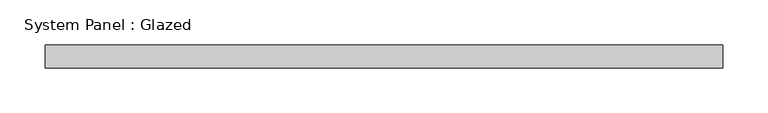
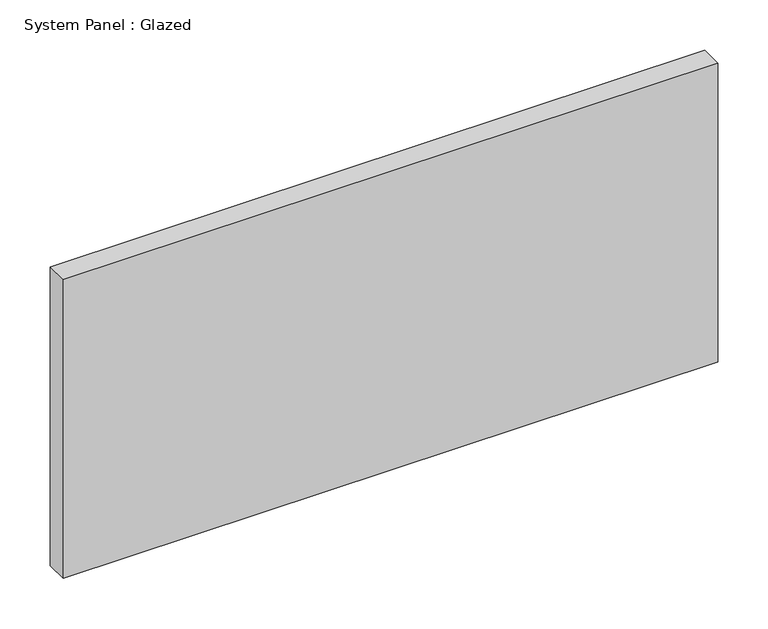
"""IFC4 building model written with IfcOpenShell, lengths in millimetres: plate geometry, System Panel : Glazed."""

from ifc_helpers import new_model, si_unit, origin, origin_with_axes, place, context, project, spatial, polyline, outline, extrude, source, transform, mapped, element, save


def system_panel_glazed_336a352b(model_context):
    return source(origin(), model_context, "Body", "SweptSolid", [
        extrude(outline(polyline([(374.65, 19.05), (-374.65, 19.05), (-374.65, 44.45), (374.65, 44.45), (374.65, 19.05)])), origin_with_axes(), (0.0, 0.0, 1.0), 361.95),
    ])


if __name__ == "__main__":
    model = new_model("IFC4")
    model_context = context("Model", 3, world=origin())
    ifc_project = project(units=[si_unit("LENGTHUNIT", "METRE", prefix="MILLI")], contexts=[model_context])
    site = spatial("IfcSite", under=ifc_project)
    building = spatial("IfcBuilding", under=site)
    placement = place(None, origin())
    system_panel_glazed_shape = system_panel_glazed_336a352b(model_context)
    element("IfcPlate", 1, ObjectType="System Panel : Glazed", at=placement, inside=building, context=model_context, shape_type="MappedRepresentation", body=[
        mapped(system_panel_glazed_shape, transform((0.0, 0.0, 0.0), x_axis=(1.0, 0.0, 0.0), y_axis=(0.0, 1.0, 0.0), z_axis=(0.0, 0.0, 1.0))),
    ])
    save(model, "model.ifc")

# Revit data of these elements
# Type "System Panel : Glazed"
#   Construction Type Id = "GSP4R"
#   Analytic Construction = "1/8 in Pilkington single glazing"
#   Visual Light Transmittance = 0.9
#   Solar Heat Gain Coefficient = 0.86
#   Heat Transfer Coefficient (U) = 1.18115 BTU/(h·ft²·°F)
#   Define Thermal Properties by = 1
# Element 1 (IfcPlate, "System Panel : Glazed")
#   Materials on its faces: "Glass"
# Materials
#   "Glass": class "Glass", colour RGB 0 128 192, transparency 0.75, Description = "Soda Lime Glass", Cost = 0
